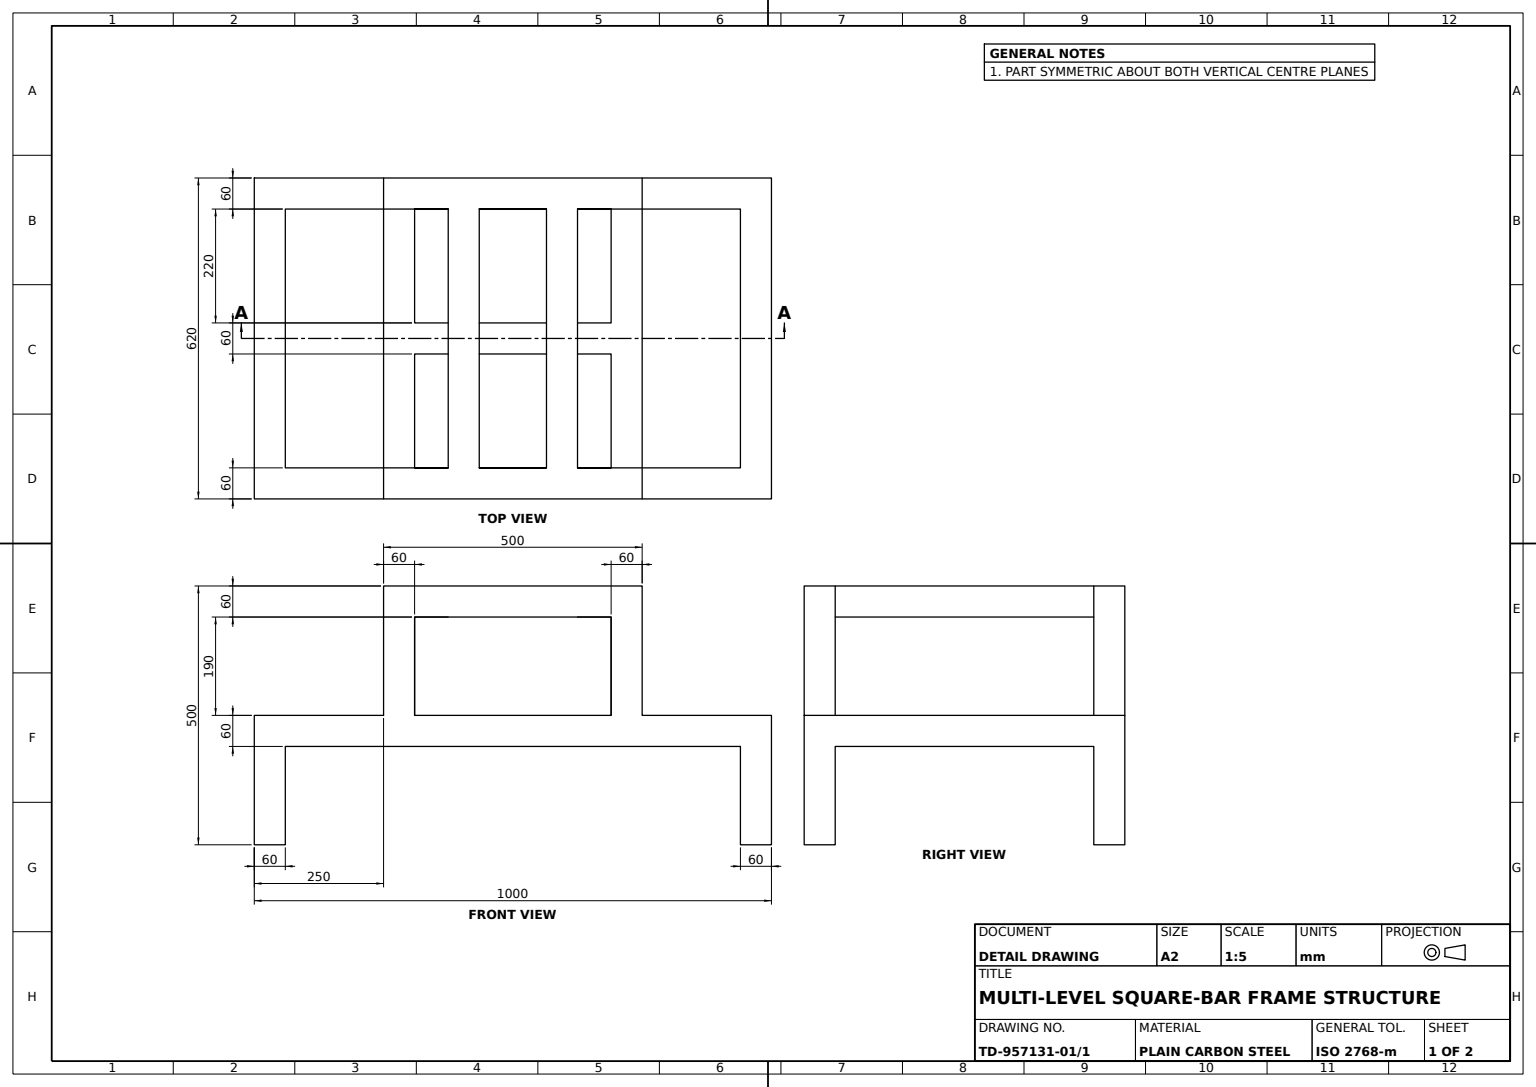
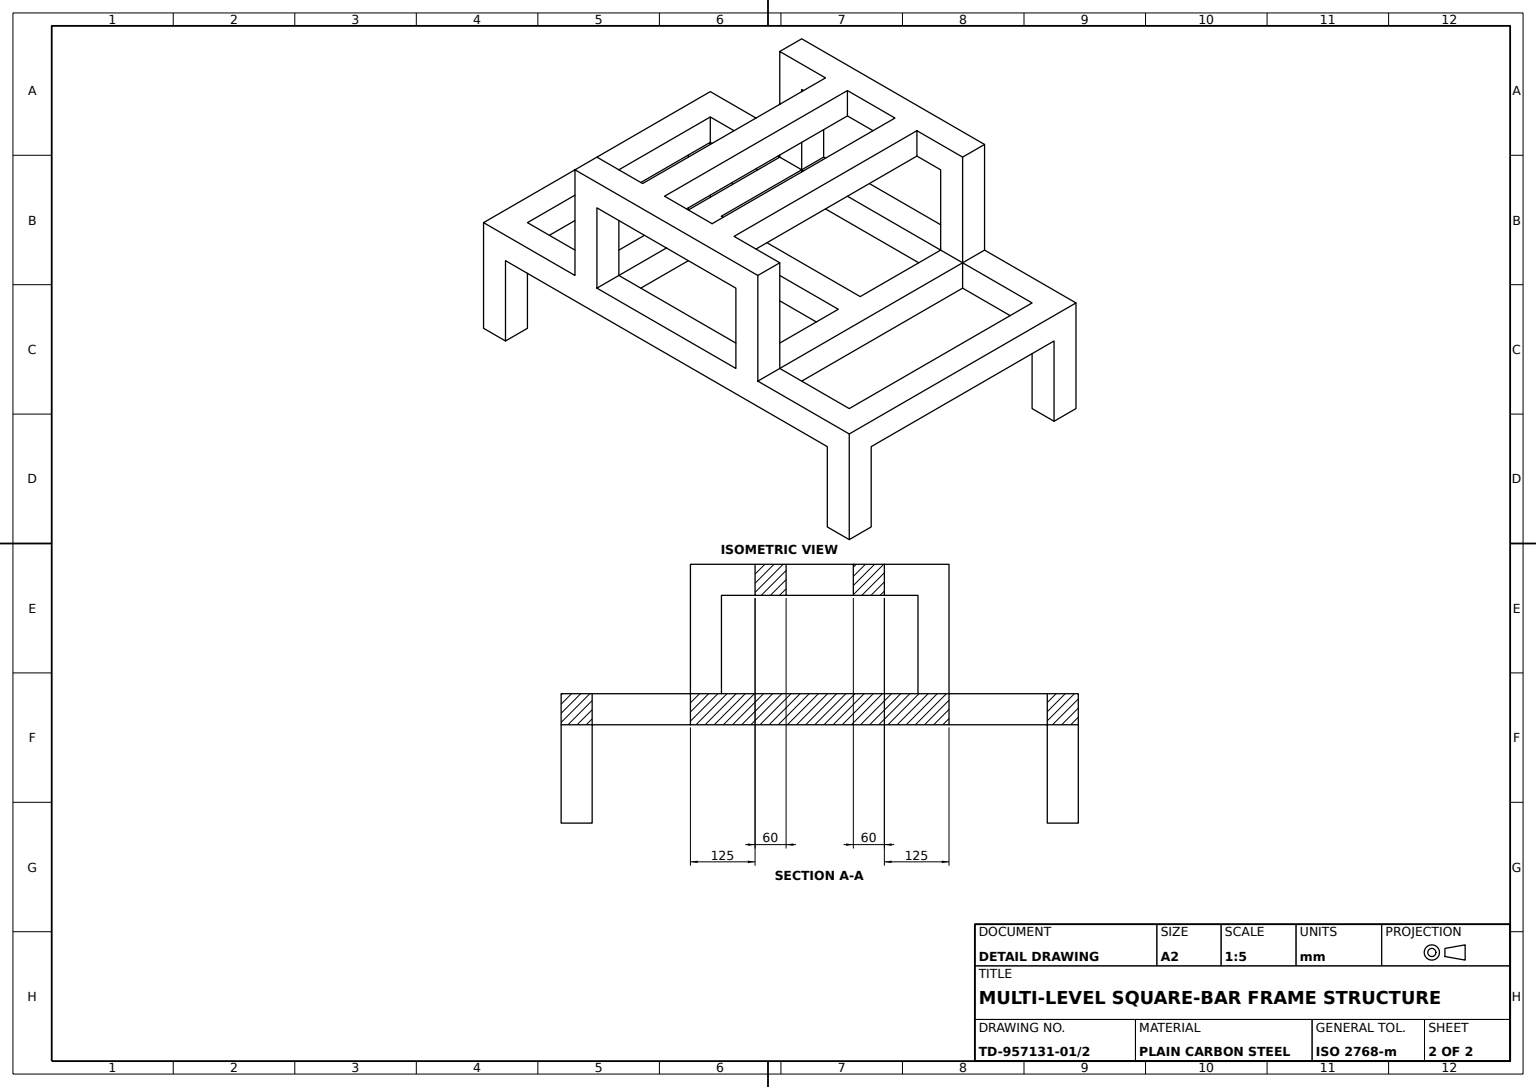
SolidWorks part; units mm, degrees
material "Plain Carbon Steel"
ref_plane "Front Plane" through (0, 0, 0) normal (0, 0, 1) x (1, 0, 0)
ref_plane "Top Plane" through (0, 0, 0) normal (0, 1, 0) x (1, 0, 0)
ref_plane "Right Plane" through (0, 0, 0) normal (1, 0, 0) x (0, 0, -1)
sketch "Front Frame Sketch" plane through (0, 0, 0) normal (0, 0, 1) x (1, 0, 0)
  line L0 (0, 0) -> (0, 250)
  line L1 (0, 250) -> (1000, 250)
  line L2 (1000, 250) -> (1000, 0)
  line L3 (0, 0) -> (60, 0)
  line L4 (60, 0) -> (60, 190)
  line L5 (1000, 0) -> (940, 0)
  line L6 (940, 0) -> (940, 190)
  line L7 (940, 190) -> (60, 190)
  dimension "D1" = 60
  dimension "D2" = 940
  dimension "D3" = 190
  dimension "D4" = 250
extrude "Front Frame" add sketch "Front Frame Sketch" along normal blind 60
sketch "Frame Member 2 Sketch" plane through (0, 250, 0) normal (0, 1, 0) x (1, 0, 0)
  line L0 (0, 0) -> (0, 500)
  line L1 (0, 500) -> (60, 500)
  line L2 (60, 500) -> (60, 0)
  line L3 (1000, 0) -> (0, 0) construction
  line L4 (60, 0) -> (0, 0)
  line L5 (1000, 0) -> (1000, 500)
  line L6 (1000, 500) -> (940, 500)
  line L7 (940, 500) -> (940, 0)
  line L8 (940, 0) -> (1000, 0)
  line L9 (0, -60) -> (0, 0) construction
  dimension "D1" = 60
  dimension "D2" = 500
extrude "Frame Member 2" add sketch "Frame Member 2 Sketch" against normal blind 60
sketch "Frame Member 3 Sketch" plane through (0, 0, -500) normal (0, 0, -1) x (-1, 0, 0)
  line L0 (-1000, 250) -> (0, 250)
  line L1 (0, 250) -> (0, 0)
  line L2 (0, 0) -> (-60, 0)
  line L3 (-60, 0) -> (-60, 190)
  line L4 (-60, 190) -> (-940, 190)
  line L5 (-940, 190) -> (-940, 0)
  line L6 (-940, 0) -> (-1000, 0)
  line L7 (-1000, 0) -> (-1000, 250)
extrude "Frame Member 3" add sketch "Frame Member 3 Sketch" along normal blind 60
sketch "Frame Member 4 Sketch" plane through (0, 0, 60) normal (0, 0, 1) x (1, 0, 0)
  line L0 (940, 190) -> (940, 0) construction
  line L1 (1000, 250) -> (0, 250) construction
  line L2 (750, 250) -> (750, 500)
  line L3 (60, 190) -> (940, 190) construction
  line L4 (250, 250) -> (250, 500)
  line L5 (250, 500) -> (750, 500)
  line L6 (250, 250) -> (310, 250)
  line L7 (750, 250) -> (690, 250)
  line L8 (690, 250) -> (690, 440)
  line L9 (690, 440) -> (310, 440)
  line L10 (310, 440) -> (310, 250)
  dimension "D1" = 190
  dimension "D2" = 250
  dimension "D3" = 630
  dimension "D4" = 250
  dimension "D5" = 310
extrude "Frame Member 4" add sketch "Frame Member 4 Sketch" against normal blind 60
sketch "Frame Member 5 Sketch" plane through (0, 0, -560) normal (0, 0, -1) x (-1, 0, 0)
  line L0 (-750, 250) -> (-750, 500)
  line L1 (-750, 500) -> (-250, 500)
  line L2 (-250, 500) -> (-250, 250)
  line L3 (-250, 250) -> (-310, 250)
  line L4 (-310, 250) -> (-310, 440)
  line L5 (-310, 440) -> (-690, 440)
  line L6 (-690, 440) -> (-690, 250)
  line L7 (-690, 250) -> (-750, 250)
extrude "Frame Member 5" add sketch "Frame Member 5 Sketch" against normal blind 60
sketch "Frame Member 6 Sketch" plane through (0, 250, 0) normal (0, 1, 0) x (1, 0, 0)
  line L0 (250, 500) -> (310, 500)
  line L1 (60, 500) -> (250, 500) construction
  line L2 (250, 500) -> (250, 560) construction
  line L3 (250, 500) -> (750, 500) construction
  line L4 (310, 500) -> (310, 0)
  line L5 (750, 0) -> (250, 0) construction
  line L6 (310, 0) -> (250, 0)
  line L7 (250, 0) -> (250, 500)
  line L8 (750, 500) -> (750, 0)
  line L9 (750, 0) -> (690, 0)
  line L10 (690, 0) -> (690, 500)
  line L11 (690, 500) -> (750, 500)
extrude "Frame Member 6" add sketch "Frame Member 6 Sketch" against normal blind 60
sketch "Frame Member 7 Sketch" plane through (0, 250, 0) normal (0, 1, 0) x (1, 0, 0)
  line L0 (310, 250) -> (310, 280)
  line L1 (310, 0) -> (310, 500) construction
  line L2 (310, 280) -> (690, 280)
  line L3 (690, 500) -> (690, 0) construction
  line L4 (690, 280) -> (690, 220)
  line L5 (690, 220) -> (310, 220)
  line L6 (310, 220) -> (310, 250)
  line L8 (250, 0) -> (310, 0) construction
  dimension "D1" = 220
extrude "Frame Member 7" add sketch "Frame Member 7 Sketch" against normal blind 60
sketch "Frame Member 8 Sketch" plane through (0, 500, 0) normal (0, 1, 0) x (1, 0, 0)
  line L0 (250, 500) -> (250, 560) construction
  line L1 (250, 500) -> (750, 500) construction
  line L2 (375, 500) -> (375, 0)
  line L3 (750, 0) -> (250, 0) construction
  line L4 (375, 0) -> (435, 0)
  line L5 (435, 0) -> (435, 500)
  line L6 (435, 500) -> (375, 500)
  line L8 (625, 0) -> (625, 500)
  line L9 (625, 500) -> (565, 500)
  line L10 (565, 500) -> (565, 0)
  line L11 (565, 0) -> (625, 0)
  dimension "D1" = 125
  dimension "D2" = 185
  dimension "D3" = 315
extrude "Frame Member 8" add sketch "Frame Member 8 Sketch" against normal blind 60
